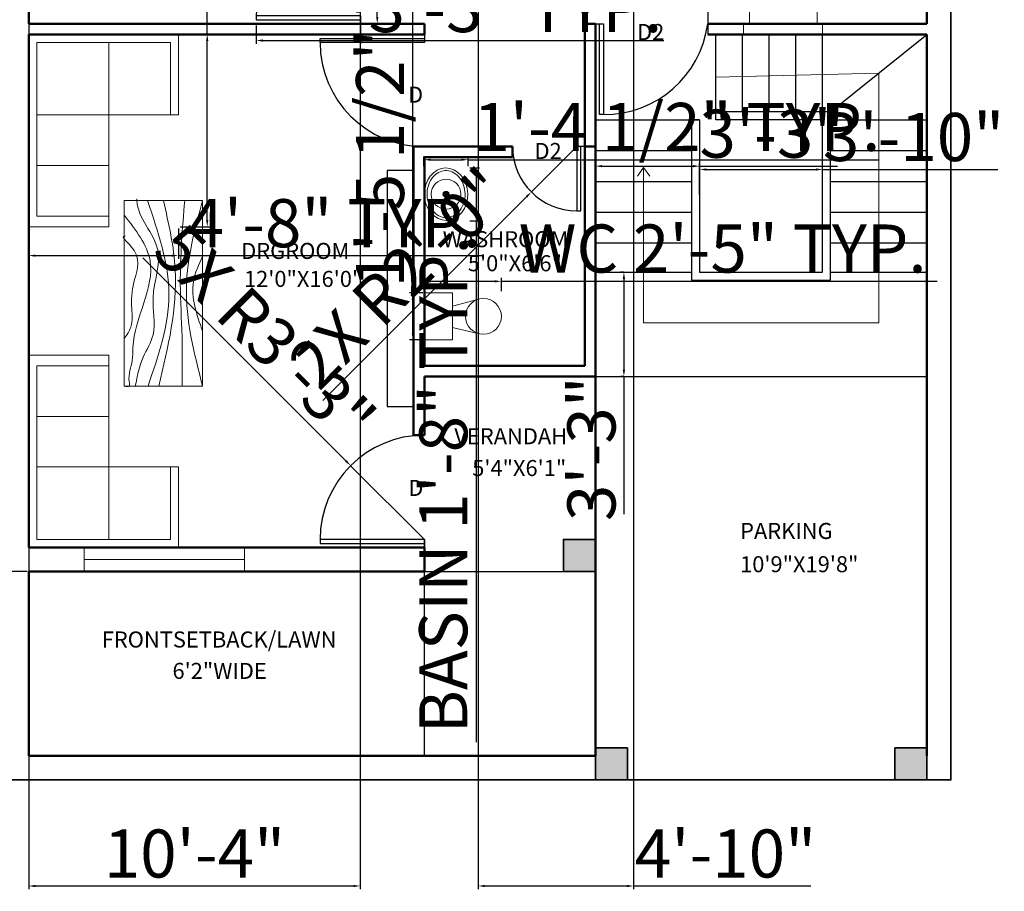
# Model space of a CAD drawing. Units: inches. Extents: x 2040 to 2729, y 1653 to 2621.
# Tile 2 of 4: x 2273 to 2641, y 1653 to 1979. Entities that reach past the tile are written whole.
import ezdxf

# ---------------------------------------------------------------- set-up
doc = ezdxf.new("R2010")
doc.units = ezdxf.units.IN
doc.layers.get('0').update_dxf_attribs({"color": 111})
for name, color, linetype, lineweight in [('A-ANNO-DIMS', 10, 'Continuous', 18), ('A-ANNO-SYMB', 10, 'Continuous', 18), ('A-ANNO-TEXT', 30, 'Continuous', 18), ('A-AREA-IDEN', 6, 'Continuous', 18), ('A-COLS', 7, 'Continuous', 35), ('A-COLS-PATT', 1, 'Continuous', 13), ('A-DOOR', 50, 'Continuous', 25), ('A-EQPM', 8, 'Continuous', 18), ('A-FLOR-CASE', 30, 'Continuous', 25), ('A-FLOR-FIXT', 4, 'Continuous', 18), ('A-FLOR-OTLN', 111, 'Continuous', 25), ('A-FLOR-STRS', 50, 'Continuous', 25), ('A-FURN', 30, 'Continuous', 18), ('A-GLAZ', 31, 'Continuous', 18), ('A-WALL', 7, 'Continuous', 50), ('C-PROP', 111, 'Continuous', 35)]:
    doc.layers.add(name, color=color, linetype=linetype, lineweight=lineweight)
doc.styles.get("Standard").update_dxf_attribs({"font": 'arial.ttf'})
doc.dimstyles.new('ISO-25', dxfattribs={"dimtxt": 18, "dimasz": 2.5, "dimexe": 1.25, "dimexo": 0.625, "dimtad": 1, "dimdec": 0, "dimlunit": 3, "dimtxsty": 'Standard', "dimcen": 2.5, "dimadec": 0, "dimazin": 0, "dimtfac": 1, "dimtdec": 0, "dimtmove": 0, "dimatfit": 3, "dimfxl": 1, "dimarcsym": 0})

# ---------------------------------------------------------------- blocks, each defined once
blk = doc.blocks.new('*D2')
at = {"layer": 'A-ANNO-DIMS', "color": 0, "lineweight": -2, "transparency": 16777216}
for p, q in [((2527.47, 1913.79), (2527.47, 1924.35)), ((2529.97, 1923.1), (2570.97, 1923.1)), ((2573.47, 1913.79), (2573.47, 1924.35)), ((2573.47, 1923.1), (2639.04, 1923.1))]:
    blk.add_line(p, q, dxfattribs=at)
at = {"layer": 'A-ANNO-DIMS', "color": 0, "transparency": 16777216}
for points in [[(2529.97, 1923.51), (2529.97, 1922.68), (2527.47, 1923.1)], [(2570.97, 1923.51), (2570.97, 1922.68), (2573.47, 1923.1)]]:
    blk.add_solid(points, dxfattribs=at)
at = {"layer": 'Defpoints', "color": 0, "transparency": 16777216}
for p in [(2573.47, 1923.1), (2527.47, 1913.16), (2573.47, 1913.16)]:
    blk.add_point(p, dxfattribs=at)
at = {"layer": 'A-ANNO-DIMS', "color": 0, "transparency": 16777216, "insert": (2607.51, 1932.92), "char_height": 18, "attachment_point": 5}
blk.add_mtext('3\'-10"', dxfattribs=at)
blk = doc.blocks.new('*D3')
at = {"layer": 'A-ANNO-DIMS', "color": 0, "lineweight": -2, "transparency": 16777216}
for p, q in [((2488.47, 1923.72), (2488.47, 1925.6)), ((2490.97, 1924.35), (2524.97, 1924.35)), ((2527.47, 1923.72), (2527.47, 1925.6)), ((2527.47, 1924.35), (2579.06, 1924.35))]:
    blk.add_line(p, q, dxfattribs=at)
at = {"layer": 'A-ANNO-DIMS', "color": 0, "transparency": 16777216}
for points in [[(2490.97, 1924.76), (2490.97, 1923.93), (2488.47, 1924.35)], [(2524.97, 1924.76), (2524.97, 1923.93), (2527.47, 1924.35)]]:
    blk.add_solid(points, dxfattribs=at)
at = {"layer": 'Defpoints', "color": 0, "transparency": 16777216}
for p in [(2488.47, 1923.1), (2527.47, 1924.35), (2527.47, 1923.1)]:
    blk.add_point(p, dxfattribs=at)
at = {"layer": 'A-ANNO-DIMS', "color": 0, "transparency": 16777216, "insert": (2554.52, 1934.17), "char_height": 18, "attachment_point": 5}
blk.add_mtext('3\'-3"', dxfattribs=at)
blk = doc.blocks.new('*D4')
at = {"layer": 'A-ANNO-DIMS', "color": 0, "lineweight": -2, "transparency": 16777216}
for p, q in [((2498.94, 1884.66), (2497.88, 1884.66)), ((2499.13, 1882.16), (2499.13, 1848.16)), ((2498.94, 1845.66), (2497.88, 1845.66)), ((2499.13, 1845.66), (2499.13, 1794.07))]:
    blk.add_line(p, q, dxfattribs=at)
at = {"layer": 'A-ANNO-DIMS', "color": 0, "transparency": 16777216}
for points in [[(2498.72, 1882.16), (2499.55, 1882.16), (2499.13, 1884.66)], [(2498.72, 1848.16), (2499.55, 1848.16), (2499.13, 1845.66)]]:
    blk.add_solid(points, dxfattribs=at)
at = {"layer": 'Defpoints', "color": 0, "transparency": 16777216}
for p in [(2499.56, 1884.66), (2499.13, 1845.66), (2499.56, 1845.66)]:
    blk.add_point(p, dxfattribs=at)
at = {"layer": 'A-ANNO-DIMS', "color": 0, "transparency": 16777216, "insert": (2489.31, 1818.62), "char_height": 18, "attachment_point": 5, "rotation": 90}
blk.add_mtext('3\'-3"', dxfattribs=at)
blk = doc.blocks.new('WC-FLOOR-MOUNT')
for p, q in [((0, 0), (10.48, 0)), ((0, -17.59), (0, 0)), ((10.48, 0), (10.48, -17.59)), ((10.48, -5), (20.35, -2.32)), ((10.48, -12.9), (20.54, -15.32)), ((10.48, -17.59), (0, -17.59))]:
    blk.add_line(p, q)
blk.add_circle((22.11, -8.8), 6.71)
blk = doc.blocks.new('BASIN-OVAL')
h = blk.add_hatch(color=256)
h.dxf.hatch_style = 1
h.paths.add_polyline_path([(1.14, 0, 1), (-1.14, 0, 1)])
for radius in [5.58, 1.14]:
    blk.add_circle((0, 0), radius)
blk.add_ellipse((0, 0), major_axis=(9.81, 0.23), ratio=0.826688)
blk.add_open_spline([(8.81, 0.21), (8.8, 0.81), (8.69, 1.4), (8.2, 2.81), (7.72, 3.6), (6.41, 5.01), (5.59, 5.62), (3.7, 6.55), (2.64, 6.87), (0.44, 7.17), (-0.7, 7.15), (-2.89, 6.76), (-3.94, 6.39), (-5.79, 5.39), (-6.59, 4.75), (-7.85, 3.29), (-8.3, 2.48), (-8.82, 0.79), (-8.88, -0.08), (-8.62, -1.78), (-8.3, -2.62), (-7.28, -4.16), (-6.59, -4.86), (-4.92, -6.01), (-3.94, -6.46), (-1.83, -7.03), (-0.7, -7.16), (1.53, -7.05), (2.64, -6.83), (4.67, -6.06), (5.59, -5.52), (7.11, -4.23), (7.72, -3.47), (8.55, -1.86), (8.78, -1), (8.82, -0.02), (8.82, 0.09), (8.81, 0.21)], degree=3, knots=[0, 0, 0, 0, 0.259704, 0.259704, 0.633026, 0.633026, 1.006347, 1.006347, 1.379668, 1.379668, 1.752989, 1.752989, 2.12631, 2.12631, 2.499631, 2.499631, 2.872952, 2.872952, 3.246274, 3.246274, 3.619595, 3.619595, 3.992916, 3.992916, 4.366237, 4.366237, 4.739558, 4.739558, 5.112879, 5.112879, 5.486201, 5.486201, 5.859522, 5.859522, 6.232843, 6.232843, 6.283185, 6.283185, 6.283185, 6.283185])
blk = doc.blocks.new('SOFA-CORNER')
for p, q in [((0, 30.1), (-55.97, 30.1)), ((-55.97, 30.1), (-55.97, -41.9)), ((0, 0), (0, 30.1)), ((-52.97, -37.9), (-52.97, 27.1)), ((-52.97, 27.1), (-2.97, 27.1)), ((-25.97, 0), (-25.97, 27.1)), ((-2.97, 27.1), (-2.97, 0)), ((-2.97, 0), (-52.97, 0)), ((-25.97, -37.9), (-25.97, 0)), ((-2.97, 0), (0, 0)), ((-25.97, -18.95), (-52.97, -18.95)), ((-25.97, -37.9), (-52.97, -37.9)), ((-25.97, -41.9), (-25.97, -37.9)), ((-55.97, -41.9), (-25.97, -41.9))]:
    blk.add_line(p, q)
blk = doc.blocks.new('DOOR-39IN')
for p, q in [((0, 0), (0, 39)), ((0, 39), (1.5, 39)), ((1.5, 39), (1.5, 0)), ((3, 0), (0, 0))]:
    blk.add_line(p, q)
blk.add_arc((0, 0), 39, 90, 180)
blk = doc.blocks.new('DOOR-39IN-ALT')
for p, q in [((0, 0), (-39, 0)), ((-39, 0), (-39, -1.5)), ((0, 0), (0, -3)), ((0, -3), (0, 0)), ((-39, -1.5), (0, -1.5)), ((-39, -1.5), (0, -1.5))]:
    blk.add_line(p, q)
blk.add_arc((0, 0), 39, 90, 180)
blk = doc.blocks.new('*D19')
at = {"layer": 'A-ANNO-DIMS', "color": 0, "lineweight": -2, "transparency": 16777216}
for p, q in [((2441.45, 1923.78), (2445.06, 1923.78)), ((2443.81, 1921.28), (2443.81, 1906.43)), ((2441.45, 1903.93), (2445.06, 1903.93)), ((2443.81, 1903.93), (2443.81, 1708.82))]:
    blk.add_line(p, q, dxfattribs=at)
at = {"layer": 'A-ANNO-DIMS', "color": 0, "transparency": 16777216}
for points in [[(2443.39, 1921.28), (2444.22, 1921.28), (2443.81, 1923.78)], [(2443.39, 1906.43), (2444.22, 1906.43), (2443.81, 1903.93)]]:
    blk.add_solid(points, dxfattribs=at)
at = {"layer": 'Defpoints', "color": 0, "transparency": 16777216}
for p in [(2440.83, 1923.78), (2440.83, 1903.93), (2443.81, 1903.93)]:
    blk.add_point(p, dxfattribs=at)
at = {"layer": 'A-ANNO-DIMS', "color": 0, "transparency": 16777216, "insert": (2433.87, 1805.12), "char_height": 18, "attachment_point": 5, "rotation": 90}
blk.add_mtext('BASIN 1\'-8" TYP.', dxfattribs=at)
blk = doc.blocks.new('*D20')
at = {"layer": 'A-ANNO-DIMS', "color": 0, "lineweight": -2, "transparency": 16777216}
for p, q in [((2424.34, 1924.4), (2424.34, 1928)), ((2426.84, 1926.75), (2438.33, 1926.75)), ((2440.83, 1924.4), (2440.83, 1928)), ((2440.83, 1926.75), (2594.55, 1926.75))]:
    blk.add_line(p, q, dxfattribs=at)
at = {"layer": 'A-ANNO-DIMS', "color": 0, "transparency": 16777216}
for points in [[(2426.84, 1927.17), (2426.84, 1926.34), (2424.34, 1926.75)], [(2438.33, 1927.17), (2438.33, 1926.34), (2440.83, 1926.75)]]:
    blk.add_solid(points, dxfattribs=at)
at = {"layer": 'Defpoints', "color": 0, "transparency": 16777216}
for p in [(2440.83, 1926.75), (2424.34, 1923.78), (2440.83, 1923.78)]:
    blk.add_point(p, dxfattribs=at)
at = {"layer": 'A-ANNO-DIMS', "color": 0, "transparency": 16777216, "insert": (2518.94, 1936.69), "char_height": 18, "attachment_point": 5}
blk.add_mtext('1\'-4 1/2" TYP.', dxfattribs=at)
blk = doc.blocks.new('*D23')
at = {"layer": 'A-ANNO-DIMS', "color": 0, "lineweight": -2, "transparency": 16777216}
for p, q in [((2424.47, 1877.55), (2424.47, 1882.49)), ((2453.3, 1877.55), (2453.3, 1882.49)), ((2426.97, 1881.24), (2450.8, 1881.24)), ((2453.3, 1881.24), (2616.39, 1881.24))]:
    blk.add_line(p, q, dxfattribs=at)
at = {"layer": 'A-ANNO-DIMS', "color": 0, "transparency": 16777216}
for points in [[(2426.97, 1881.66), (2426.97, 1880.83), (2424.47, 1881.24)], [(2450.8, 1881.66), (2450.8, 1880.83), (2453.3, 1881.24)]]:
    blk.add_solid(points, dxfattribs=at)
at = {"layer": 'Defpoints', "color": 0, "transparency": 16777216}
for p in [(2453.3, 1881.24), (2424.47, 1876.92), (2453.3, 1876.92)]:
    blk.add_point(p, dxfattribs=at)
at = {"layer": 'A-ANNO-DIMS', "color": 0, "transparency": 16777216, "insert": (2536.09, 1891.18), "char_height": 18, "attachment_point": 5}
blk.add_mtext('WC 2\'-5" TYP.', dxfattribs=at)
blk = doc.blocks.new('*D24')
at = {"layer": 'A-ANNO-DIMS', "color": 0, "lineweight": -2, "transparency": 16777216}
for p, q in [((2420.15, 1876.92), (2420.15, 2030.64)), ((2423.85, 1876.92), (2418.9, 1876.92)), ((2420.15, 1861.83), (2420.15, 1874.42)), ((2423.85, 1859.33), (2418.9, 1859.33))]:
    blk.add_line(p, q, dxfattribs=at)
at = {"layer": 'A-ANNO-DIMS', "color": 0, "transparency": 16777216}
for points in [[(2419.73, 1874.42), (2420.57, 1874.42), (2420.15, 1876.92)], [(2419.73, 1861.83), (2420.57, 1861.83), (2420.15, 1859.33)]]:
    blk.add_solid(points, dxfattribs=at)
at = {"layer": 'Defpoints', "color": 0, "transparency": 16777216}
for p in [(2420.15, 1876.92), (2424.47, 1876.92), (2424.47, 1859.33)]:
    blk.add_point(p, dxfattribs=at)
at = {"layer": 'A-ANNO-DIMS', "color": 0, "transparency": 16777216, "insert": (2410.22, 1955.03), "char_height": 18, "attachment_point": 5, "rotation": 90}
blk.add_mtext('1\'-5 1/2" TYP.', dxfattribs=at)
blk = doc.blocks.new('*D29')
at = {"layer": 'A-ANNO-DIMS', "color": 0, "lineweight": -2, "transparency": 16777216}
for p, q in [((2343.24, 1973.66), (2343.24, 2162.49)), ((2333.07, 1973.66), (2344.49, 1973.66)), ((2343.24, 1904.16), (2343.24, 1971.16)), ((2333.07, 1901.66), (2344.49, 1901.66))]:
    blk.add_line(p, q, dxfattribs=at)
at = {"layer": 'A-ANNO-DIMS', "color": 0, "transparency": 16777216}
for points in [[(2342.83, 1971.16), (2343.66, 1971.16), (2343.24, 1973.66)], [(2342.83, 1904.16), (2343.66, 1904.16), (2343.24, 1901.66)]]:
    blk.add_solid(points, dxfattribs=at)
at = {"layer": 'Defpoints', "color": 0, "transparency": 16777216}
for p in [(2332.44, 1973.66), (2343.24, 1973.66), (2332.44, 1901.66)]:
    blk.add_point(p, dxfattribs=at)
at = {"layer": 'A-ANNO-DIMS', "color": 0, "transparency": 16777216, "insert": (2333.3, 2069.33), "char_height": 18, "attachment_point": 5, "rotation": 90}
blk.add_mtext('SOFA 6\'-0" TYP.', dxfattribs=at)
blk = doc.blocks.new('*D30')
at = {"layer": 'A-ANNO-DIMS', "color": 0, "lineweight": -2, "transparency": 16777216}
for p, q in [((2276.47, 1901.04), (2276.47, 1889.61)), ((2332.44, 1901.04), (2332.44, 1889.61)), ((2278.97, 1890.86), (2329.94, 1890.86)), ((2332.44, 1890.86), (2446.64, 1890.86))]:
    blk.add_line(p, q, dxfattribs=at)
at = {"layer": 'A-ANNO-DIMS', "color": 0, "transparency": 16777216}
for points in [[(2278.97, 1891.28), (2278.97, 1890.44), (2276.47, 1890.86)], [(2329.94, 1891.28), (2329.94, 1890.44), (2332.44, 1890.86)]]:
    blk.add_solid(points, dxfattribs=at)
at = {"layer": 'Defpoints', "color": 0, "transparency": 16777216}
for p in [(2276.47, 1901.66), (2332.44, 1901.66), (2332.44, 1890.86)]:
    blk.add_point(p, dxfattribs=at)
at = {"layer": 'A-ANNO-DIMS', "color": 0, "transparency": 16777216, "insert": (2390.79, 1900.68), "char_height": 18, "attachment_point": 5}
blk.add_mtext('4\'-8" TYP.', dxfattribs=at)
blk = doc.blocks.new('*D33')
at = {"layer": 'A-ANNO-DIMS', "color": 0, "lineweight": -2, "transparency": 16777216}
for p, q in [((2406.86, 2019.66), (2406.86, 2351.67)), ((2401.19, 2019.66), (2408.11, 2019.66)), ((2406.86, 1980.16), (2406.86, 2017.16)), ((2401.19, 1977.66), (2408.11, 1977.66))]:
    blk.add_line(p, q, dxfattribs=at)
at = {"layer": 'A-ANNO-DIMS', "color": 0, "transparency": 16777216}
for points in [[(2406.45, 2017.16), (2407.28, 2017.16), (2406.86, 2019.66)], [(2406.45, 1980.16), (2407.28, 1980.16), (2406.86, 1977.66)]]:
    blk.add_solid(points, dxfattribs=at)
at = {"layer": 'Defpoints', "color": 0, "transparency": 16777216}
for p in [(2400.56, 2019.66), (2406.86, 2019.66), (2400.56, 1977.66)]:
    blk.add_point(p, dxfattribs=at)
at = {"layer": 'A-ANNO-DIMS', "color": 0, "transparency": 16777216, "insert": (2396.92, 2186.92), "char_height": 18, "attachment_point": 5, "rotation": 90}
blk.add_mtext('BEDROOM DOOR 3\'-6" TYP.', dxfattribs=at)
blk = doc.blocks.new('*D34')
at = {"layer": 'A-ANNO-DIMS', "color": 0, "lineweight": -2, "transparency": 16777216}
for p, q in [((2361.56, 1977.04), (2361.56, 1970.11)), ((2400.56, 1977.04), (2400.56, 1970.11)), ((2364.06, 1971.36), (2398.06, 1971.36)), ((2400.56, 1971.36), (2514.02, 1971.36))]:
    blk.add_line(p, q, dxfattribs=at)
at = {"layer": 'A-ANNO-DIMS', "color": 0, "transparency": 16777216}
for points in [[(2364.06, 1971.78), (2364.06, 1970.94), (2361.56, 1971.36)], [(2398.06, 1971.78), (2398.06, 1970.94), (2400.56, 1971.36)]]:
    blk.add_solid(points, dxfattribs=at)
at = {"layer": 'Defpoints', "color": 0, "transparency": 16777216}
for p in [(2361.56, 1977.66), (2400.56, 1977.66), (2400.56, 1971.36)]:
    blk.add_point(p, dxfattribs=at)
at = {"layer": 'A-ANNO-DIMS', "color": 0, "transparency": 16777216, "insert": (2458.54, 1981.18), "char_height": 18, "attachment_point": 5}
blk.add_mtext('3\'-3" TYP.', dxfattribs=at)
blk = doc.blocks.new('*D41')
at = {"layer": 'A-ANNO-DIMS', "color": 0, "lineweight": -2, "transparency": 16777216}
for p, q in [((2266.85, 2402.66), (2226.49, 2402.66)), ((2227.74, 1775.16), (2227.74, 2400.16)), ((2275.85, 1772.66), (2226.49, 1772.66))]:
    blk.add_line(p, q, dxfattribs=at)
at = {"layer": 'A-ANNO-DIMS', "color": 0, "transparency": 16777216}
for points in [[(2227.33, 2400.16), (2228.16, 2400.16), (2227.74, 2402.66)], [(2227.33, 1775.16), (2228.16, 1775.16), (2227.74, 1772.66)]]:
    blk.add_solid(points, dxfattribs=at)
at = {"layer": 'Defpoints', "color": 0, "transparency": 16777216}
for p in [(2227.74, 2402.66), (2267.47, 2402.66), (2276.47, 1772.66)]:
    blk.add_point(p, dxfattribs=at)
at = {"layer": 'A-ANNO-DIMS', "color": 0, "transparency": 16777216, "insert": (2217.93, 2087.66), "char_height": 18, "attachment_point": 5, "rotation": 90}
blk.add_mtext('52\'-6"', dxfattribs=at)
blk = doc.blocks.new('*D44')
at = {"layer": 'A-ANNO-DIMS', "color": 0, "lineweight": -2, "transparency": 16777216}
for p, q in [((2276.47, 2169.04), (2276.47, 1653.68)), ((2400.47, 2169.04), (2400.47, 1653.68)), ((2278.97, 1654.93), (2397.97, 1654.93))]:
    blk.add_line(p, q, dxfattribs=at)
at = {"layer": 'A-ANNO-DIMS', "color": 0, "transparency": 16777216}
for points in [[(2278.97, 1655.35), (2278.97, 1654.51), (2276.47, 1654.93)], [(2397.97, 1655.35), (2397.97, 1654.51), (2400.47, 1654.93)]]:
    blk.add_solid(points, dxfattribs=at)
at = {"layer": 'Defpoints', "color": 0, "transparency": 16777216}
for p in [(2276.47, 2169.66), (2400.47, 2169.66), (2400.47, 1654.93)]:
    blk.add_point(p, dxfattribs=at)
at = {"layer": 'A-ANNO-DIMS', "color": 0, "transparency": 16777216, "insert": (2338.47, 1664.75), "char_height": 18, "attachment_point": 5}
blk.add_mtext('10\'-4"', dxfattribs=at)
blk = doc.blocks.new('*D45')
at = {"layer": 'A-ANNO-DIMS', "color": 0, "lineweight": -2, "transparency": 16777216}
for p, q in [((2444.6, 2057.89), (2444.6, 1653.68)), ((2502.75, 2057.89), (2502.75, 1653.68)), ((2447.1, 1654.93), (2500.25, 1654.93)), ((2502.75, 1654.93), (2569.05, 1654.93))]:
    blk.add_line(p, q, dxfattribs=at)
at = {"layer": 'A-ANNO-DIMS', "color": 0, "transparency": 16777216}
for points in [[(2447.1, 1655.35), (2447.1, 1654.51), (2444.6, 1654.93)], [(2500.25, 1655.35), (2500.25, 1654.51), (2502.75, 1654.93)]]:
    blk.add_solid(points, dxfattribs=at)
at = {"layer": 'Defpoints', "color": 0, "transparency": 16777216}
for p in [(2444.6, 2058.52), (2502.75, 2058.52), (2502.75, 1654.93)]:
    blk.add_point(p, dxfattribs=at)
at = {"layer": 'A-ANNO-DIMS', "color": 0, "transparency": 16777216, "insert": (2537.15, 1664.75), "char_height": 18, "attachment_point": 5}
blk.add_mtext('4\'-10"', dxfattribs=at)
blk = doc.blocks.new('*D48')
at = {"layer": 'A-ANNO-DIMS', "color": 0, "lineweight": -2, "transparency": 16777216}
for p, q in [((2481.47, 1931.66), (2464.5, 1914.69)), ((2386.5, 1836.69), (2462.74, 1912.92))]:
    blk.add_line(p, q, dxfattribs=at)
at = {"layer": 'A-ANNO-DIMS', "color": 0, "transparency": 16777216}
blk.add_solid([(2462.44, 1913.22), (2463.03, 1912.63), (2464.5, 1914.69)], dxfattribs=at)
at = {"layer": 'Defpoints', "color": 0, "transparency": 16777216}
for p in [(2481.47, 1931.66), (2464.5, 1914.69)]:
    blk.add_point(p, dxfattribs=at)
at = {"layer": 'A-ANNO-DIMS', "color": 0, "transparency": 16777216, "insert": (2416.79, 1880.86), "char_height": 18, "attachment_point": 5, "rotation": 44.9992}
blk.add_mtext('2X R2\'-0"', dxfattribs=at)
blk = doc.blocks.new('*D52')
at = {"layer": 'A-ANNO-DIMS', "color": 0, "lineweight": -2, "transparency": 16777216}
for p, q in [((2319.12, 1890.03), (2395.13, 1814.01)), ((2424.47, 1784.66), (2396.9, 1812.24))]:
    blk.add_line(p, q, dxfattribs=at)
at = {"layer": 'A-ANNO-DIMS', "color": 0, "transparency": 16777216}
blk.add_solid([(2395.43, 1814.3), (2394.84, 1813.71), (2396.9, 1812.24)], dxfattribs=at)
at = {"layer": 'Defpoints', "color": 0, "transparency": 16777216}
for p in [(2396.9, 1812.24), (2424.47, 1784.66)]:
    blk.add_point(p, dxfattribs=at)
at = {"layer": 'A-ANNO-DIMS', "color": 0, "transparency": 16777216, "insert": (2363.19, 1859.85), "char_height": 18, "attachment_point": 5, "rotation": 314.9947}
blk.add_mtext('5X R3\'-3"', dxfattribs=at)

msp = doc.modelspace()

# ---------------------------------------------------------------- hatches: boundary and pattern name
at = {"layer": 'A-COLS-PATT'}
h = msp.add_hatch(color=256, dxfattribs=at)
h.dxf.hatch_style = 1
h.paths.add_polyline_path([(2488.47, 1784.66), (2476.47, 1784.66), (2476.47, 1772.66), (2488.47, 1772.66)])
h = msp.add_hatch(color=256, dxfattribs=at)
h.dxf.hatch_style = 1
h.paths.add_polyline_path([(2500.47, 1706.66), (2488.47, 1706.66), (2488.47, 1703.66), (2488.47, 1694.66), (2500.47, 1694.66)])
h = msp.add_hatch(color=256, dxfattribs=at)
h.dxf.hatch_style = 1
h.paths.add_polyline_path([(2612.47, 1703.66), (2612.47, 1706.66), (2600.47, 1706.66), (2600.47, 1694.66), (2612.47, 1694.66)])

# ---------------------------------------------------------------- linework, layer by layer
at = {"layer": 'A-ANNO-SYMB'}
for p, q in [((2533.47, 1957.66), (2594.47, 1959.16)), ((2594.47, 1959.16), (2594.47, 1865.68)), ((2506.47, 1923.9), (2504.18, 1920.62)), ((2506.47, 1865.68), (2506.47, 1923.9)), ((2506.47, 1923.9), (2508.77, 1920.62)), ((2594.47, 1865.68), (2506.47, 1865.68))]:
    msp.add_line(p, q, dxfattribs=at)
at = {"layer": 'A-COLS'}
for p, q in [((2500.47, 1706.66), (2488.47, 1706.66)), ((2500.47, 1694.66), (2500.47, 1706.66)), ((2600.47, 1694.66), (2600.47, 1706.66)), ((2600.47, 1706.66), (2612.47, 1706.66)), ((2488.47, 1703.66), (2488.47, 1694.66)), ((2612.47, 1703.66), (2612.47, 1694.66)), ((2488.47, 1694.66), (2500.47, 1694.66)), ((2612.47, 1694.66), (2600.47, 1694.66))]:
    msp.add_line(p, q, dxfattribs=at)
msp.add_lwpolyline([(2488.47, 1772.66), (2476.47, 1772.66), (2476.47, 1784.66), (2488.47, 1784.66)], close=True, dxfattribs=at)
at = {"layer": 'A-DOOR'}
for p, q in [((2488.47, 1977.66), (2491.47, 1977.66)), ((2489.97, 1943.66), (2489.97, 1977.66)), ((2491.47, 1977.66), (2491.47, 1943.66)), ((2491.47, 1943.66), (2489.97, 1943.66)), ((2484.47, 1931.66), (2481.47, 1931.66)), ((2481.47, 1931.66), (2481.47, 1907.66)), ((2482.97, 1907.66), (2482.97, 1931.66)), ((2481.47, 1907.66), (2482.97, 1907.66))]:
    msp.add_line(p, q, dxfattribs=at)
for centre, radius, start, end in [((2491.8, 1982.66), 39, 269.5274, 352.6361), ((2481.47, 1931.66), 24, 180, 270)]:
    msp.add_arc(centre, radius, start, end, dxfattribs=at)
at = {"layer": 'A-EQPM'}
msp.add_lwpolyline([(2571.47, 1977.66), (2546.15, 1977.66), (2546.15, 2001.66), (2571.47, 2001.66)], close=True, dxfattribs=at)
at = {"layer": 'A-FLOR-CASE'}
msp.add_line((2530.47, 2001.66), (2530.47, 1973.66), dxfattribs=at)
msp.add_lwpolyline([(2420.47, 1922.66), (2410.6, 1922.66), (2410.6, 1834.33), (2420.47, 1834.33)], close=True, dxfattribs=at)
at = {"layer": 'A-FLOR-OTLN'}
for p, q in [((2424.47, 1703.66), (2424.47, 1772.66)), ((2424.47, 1772.66), (2488.47, 1772.66))]:
    msp.add_line(p, q, dxfattribs=at)
at = {"layer": 'A-FLOR-STRS'}
for p, q in [((2533.47, 1941.66), (2533.47, 1973.66)), ((2543.47, 1944.66), (2543.47, 1973.66)), ((2553.47, 1944.66), (2553.47, 1973.66)), ((2563.47, 1944.66), (2563.47, 1973.66)), ((2573.47, 1944.66), (2573.47, 1973.66)), ((2576.47, 1944.66), (2612.47, 1973.66)), ((2488.47, 1941.66), (2527.47, 1941.66)), ((2527.47, 1941.66), (2524.47, 1941.66)), ((2524.47, 1941.66), (2524.47, 1881.66)), ((2527.47, 1941.66), (2527.47, 1884.66)), ((2576.47, 1944.66), (2533.47, 1944.66)), ((2573.47, 1941.66), (2533.47, 1941.66)), ((2573.47, 1884.66), (2573.47, 1941.66)), ((2576.47, 1881.66), (2576.47, 1944.66)), ((2576.47, 1941.66), (2612.47, 1941.66)), ((2488.47, 1930.16), (2524.47, 1930.16)), ((2576.47, 1930.16), (2612.47, 1930.16)), ((2488.47, 1918.66), (2524.47, 1918.66)), ((2576.47, 1918.66), (2612.47, 1918.66)), ((2488.47, 1907.16), (2524.47, 1907.16)), ((2576.47, 1907.16), (2612.47, 1907.16)), ((2488.47, 1895.66), (2524.47, 1895.66)), ((2576.47, 1895.66), (2612.47, 1895.66)), ((2488.47, 1884.66), (2524.47, 1884.66)), ((2527.47, 1884.66), (2573.47, 1884.66)), ((2576.47, 1884.66), (2612.47, 1884.66)), ((2524.47, 1881.66), (2576.47, 1881.66)), ((2488.47, 1845.66), (2612.47, 1845.66))]:
    msp.add_line(p, q, dxfattribs=at)
at = {"layer": 'A-FURN'}
msp.add_line((2332.44, 1781.66), (2276.47, 1781.66), dxfattribs=at)
msp.add_lwpolyline([(2312.21, 1911.49), (2341.5, 1911.49), (2341.5, 1842.04), (2312.21, 1842.04)], close=True, dxfattribs=at)
for points, knots in [([(2316.32, 1842.04), (2317.07, 1845.73), (2318.42, 1852.4), (2324.92, 1862.47), (2321.12, 1876.55), (2329.02, 1894.28), (2316.88, 1905.01), (2316.95, 1911.91), (2316.95, 1912.13)], [0, 0, 0, 0, 11.286534, 20.351276, 34.306788, 52.246482, 72.293035, 72.936945, 72.936945, 72.936945, 72.936945]), ([(2320.85, 1911.49), (2324.89, 1899.76), (2332.87, 1876.61), (2324.99, 1853.46), (2321.1, 1842.04)], [0, 0, 0, 0, 36.097508, 71.234431, 71.234431, 71.234431, 71.234431]), ([(2326.85, 1911.49), (2328.84, 1902.86), (2334.15, 1879.8), (2328.6, 1856.58), (2325.13, 1842.04)], [0, 0, 0, 0, 26.261914, 70.259672, 70.259672, 70.259672, 70.259672]), ([(2334.82, 1911.49), (2333.96, 1901.1), (2332.56, 1884.14), (2334.04, 1860.98), (2333.89, 1848.22), (2333.81, 1842.04)], [0, 0, 0, 0, 31.207497, 50.956396, 69.500686, 69.500686, 69.500686, 69.500686]), ([(2341.5, 1911.49), (2338.6, 1900.73), (2332.38, 1877.65), (2338.32, 1854.43), (2341.5, 1842.04)], [0, 0, 0, 0, 32.857913, 70.498944, 70.498944, 70.498944, 70.498944]), ([(2312.21, 1905.97), (2316.51, 1900.44), (2328.12, 1885.51), (2314.88, 1866.09), (2315.54, 1850.39), (2313.37, 1846.4), (2314.49, 1841.56), (2312.99, 1841.87), (2312.21, 1842.04)], [0, 0, 0, 0, 19.52057, 52.709722, 57.61946, 65.496264, 67.193354, 69.034395, 69.034395, 69.034395, 69.034395]), ([(2312.21, 1859.83), (2313.2, 1861.21), (2315.79, 1864.84), (2314.46, 1872.84), (2315.8, 1883.1), (2319.4, 1890.8), (2310.78, 1898.23), (2312.43, 1898.18), (2312.54, 1898.17)], [0, 0, 0, 0, 4.937051, 12.987406, 22.85915, 35.522025, 39.856714, 40.187852, 40.187852, 40.187852, 40.187852]), ([(2341.5, 1890.63), (2340.06, 1887.51), (2335.91, 1878.51), (2339.29, 1868.88), (2341.5, 1862.59)], [0, 0, 0, 0, 10.026259, 28.943072, 28.943072, 28.943072, 28.943072])]:
    msp.add_open_spline(points, degree=3, knots=knots, dxfattribs=at)
at = {"layer": 'A-GLAZ'}
msp.add_line((2297.24, 1777.16), (2357.24, 1777.16), dxfattribs=at)
for points in [[(2543.91, 1977.66), (2573.47, 1977.66), (2573.47, 1973.66), (2543.91, 1973.66)], [(2297.24, 1781.66), (2357.24, 1781.66), (2357.24, 1772.66), (2297.24, 1772.66)]]:
    msp.add_lwpolyline(points, close=True, dxfattribs=at)
at = {"layer": 'A-WALL'}
for p, q in [((2276.47, 1977.66), (2276.47, 2393.66)), ((2612.47, 2121.66), (2612.47, 1977.66)), ((2276.47, 1977.66), (2424.47, 1977.66)), ((2424.47, 1973.66), (2424.47, 1977.66)), ((2484.47, 1849.66), (2484.47, 1977.66)), ((2484.47, 1977.66), (2488.47, 1977.66)), ((2488.47, 1703.66), (2488.47, 1977.66)), ((2530.47, 1977.66), (2612.47, 1977.66)), ((2276.47, 1973.66), (2424.47, 1973.66)), ((2276.47, 1781.66), (2276.47, 1973.66)), ((2530.47, 1973.66), (2612.47, 1973.66)), ((2612.47, 1973.66), (2612.47, 1703.66)), ((2420.47, 1931.66), (2457.47, 1931.66)), ((2420.47, 1922.66), (2420.47, 1931.66)), ((2457.47, 1931.66), (2457.47, 1927.66)), ((2484.47, 1931.66), (2488.47, 1931.66)), ((2424.47, 1927.66), (2457.47, 1927.66)), ((2424.47, 1918.66), (2424.47, 1927.66)), ((2420.47, 1823.66), (2420.47, 1922.66)), ((2424.47, 1849.66), (2424.47, 1918.66)), ((2424.47, 1849.66), (2484.47, 1849.66)), ((2424.47, 1823.66), (2424.47, 1845.66)), ((2424.47, 1845.66), (2488.47, 1845.66)), ((2424.47, 1823.66), (2420.47, 1823.66)), ((2276.47, 1781.66), (2424.47, 1781.66)), ((2424.47, 1781.66), (2424.47, 1772.66)), ((2276.47, 1703.66), (2276.47, 1772.66)), ((2424.47, 1772.66), (2276.47, 1772.66)), ((2488.47, 1703.66), (2276.47, 1703.66))]:
    msp.add_line(p, q, dxfattribs=at)
at = {"layer": 'C-PROP'}
msp.add_lwpolyline([(2267.47, 2402.66), (2621.47, 2402.66), (2621.47, 1694.66), (2267.47, 1694.66)], close=True, dxfattribs=at)

# ---------------------------------------------------------------- block references
at = {"layer": 'A-DOOR'}
for p in [(2400.56, 1980.66), (2424.47, 1784.66)]:
    msp.add_blockref('DOOR-39IN-ALT', p, dxfattribs=at)
at = {"layer": 'A-DOOR', "rotation": 89.99999999999785}
msp.add_blockref('DOOR-39IN', (2424.47, 1970.66), dxfattribs=at)
at = {"layer": 'A-FLOR-FIXT', "rotation": 269.9999999999998}
msp.add_blockref('BASIN-OVAL', (2432.59, 1913.86), dxfattribs=at)
at = {"layer": 'A-FLOR-FIXT'}
msp.add_blockref('WC-FLOOR-MOUNT', (2424.47, 1876.92), dxfattribs=at)
at = {"layer": 'A-FURN'}
msp.add_blockref('SOFA-CORNER', (2332.44, 1943.56), dxfattribs=at)
at = {"layer": 'A-FURN', "extrusion": (0, 0, -1), "zscale": -1, "rotation": 180}
msp.add_blockref('SOFA-CORNER', (-2332.44, 1811.76), dxfattribs=at)

# ---------------------------------------------------------------- texts
at = {"layer": 'A-ANNO-TEXT'}
for tag, p in [('D2', (2504.06, 1971.54)), ('D', (2418.38, 1948.11)), ('D2', (2465.69, 1927.03)), ('D', (2418.5, 1800.92))]:
    msp.add_attdef(tag, p, '', height=6, dxfattribs=at)
at = {"layer": 'A-AREA-IDEN'}
for tag, p in [('WASHROOM', (2431.34, 1894.01)), ('DRGROOM', (2355.96, 1889.62)), ('5\'0"X6\'6"', (2440.76, 1885.01)), ('12\'0"X16\'0"', (2357, 1879.15)), ('VERANDAH', (2435.7, 1820.27)), ('5\'4"X6\'1"', (2442.38, 1808.36)), ('PARKING', (2542.61, 1784.81)), ('10\'9"X19\'8"', (2542.61, 1772.37)), ('FRONTSETBACK/LAWN', (2303.78, 1744.19)), ('6\'2"WIDE', (2330.24, 1732.44))]:
    msp.add_attdef(tag, p, '', height=6, dxfattribs=at)

# ---------------------------------------------------------------- dimensions: what is measured, and where the dimension line sits
at = {"layer": 'A-ANNO-DIMS'}
for base, p1, p2, override, picture, middle in [((2227.74, 2402.66), (2276.47, 1772.66), (2267.47, 2402.66), {"dimdec": 1, "dimlfac": 1, "dimrnd": 0, "dimzin": 1, "dimdsep": 46, "dimlunit": 4, "dimfrac": 2}, '*D41', (2217.93, 2087.66)), ((2499.13, 1845.66), (2499.56, 1884.66), (2499.56, 1845.66), {"dimclrd": 0, "dimclre": 0, "dimclrt": 0}, '*D4', (2489.31, 1818.62))]:
    dim = msp.add_linear_dim(base=base, p1=p1, p2=p2, angle=90, dimstyle='ISO-25', override=override, dxfattribs=at)
    dim.commit()
    dim.dimension.update_dxf_attribs({"geometry": picture, "text_midpoint": middle})
for base, p1, p2, angle, text, picture, middle in [((2406.86, 2019.66), (2400.56, 1977.66), (2400.56, 2019.66), 90, 'BEDROOM DOOR <> TYP.', '*D33', (2396.92, 2186.92)), ((2343.24, 1973.66), (2332.44, 1901.66), (2332.44, 1973.66), 90, 'SOFA <> TYP.', '*D29', (2333.3, 2069.33)), ((2420.15, 1876.92), (2424.47, 1859.33), (2424.47, 1876.92), 90, '<> TYP.', '*D24', (2410.22, 1955.03)), ((2443.8059, 1903.9348), (2440.8296, 1923.7768), (2440.8296, 1903.9348), 270, 'BASIN <> TYP.', '*D19', (2433.8739, 1805.1249))]:
    dim = msp.add_linear_dim(base=base, p1=p1, p2=p2, angle=angle, text=text, dimstyle='ISO-25', override={"dimdec": 1, "dimlfac": 1, "dimrnd": 0, "dimzin": 1, "dimdsep": 46, "dimlunit": 4, "dimfrac": 2}, dxfattribs=at)
    dim.commit()
    dim.dimension.update_dxf_attribs({"geometry": picture, "text_midpoint": middle})
for base, p1, p2, override, picture, middle in [((2400.47, 1654.93), (2276.47, 2169.66), (2400.47, 2169.66), {"dimdec": 1, "dimlfac": 1, "dimrnd": 0, "dimzin": 1, "dimdsep": 46, "dimlunit": 4, "dimfrac": 2}, '*D44', (2338.47, 1664.75)), ((2502.7465, 1654.9312), (2444.5957, 2058.5173), (2502.7465, 2058.5173), {"dimdec": 1, "dimlfac": 1, "dimrnd": 0, "dimzin": 1, "dimdsep": 46, "dimlunit": 4, "dimfrac": 2}, '*D45', (2537.1505, 1664.7465)), ((2527.47, 1924.35), (2488.47, 1923.1), (2527.47, 1923.1), {"dimclrd": 0, "dimclre": 0, "dimclrt": 0}, '*D3', (2554.52, 1934.17)), ((2573.47, 1923.1), (2527.47, 1913.16), (2573.47, 1913.16), {"dimclrd": 0, "dimclre": 0, "dimclrt": 0}, '*D2', (2607.51, 1932.92))]:
    dim = msp.add_linear_dim(base=base, p1=p1, p2=p2, dimstyle='ISO-25', override=override, dxfattribs=at)
    dim.commit()
    dim.dimension.update_dxf_attribs({"geometry": picture, "text_midpoint": middle})
for base, p1, p2, text, picture, middle in [((2400.56, 1971.36), (2361.56, 1977.66), (2400.56, 1977.66), '<> TYP.', '*D34', (2458.54, 1981.18)), ((2440.83, 1926.75), (2424.34, 1923.78), (2440.83, 1923.78), '<> TYP.', '*D20', (2518.94, 1936.69)), ((2453.3, 1881.24), (2424.47, 1876.92), (2453.3, 1876.92), 'WC <> TYP.', '*D23', (2536.09, 1891.18)), ((2332.44, 1890.86), (2276.47, 1901.66), (2332.44, 1901.66), '<> TYP.', '*D30', (2390.79, 1900.68))]:
    dim = msp.add_linear_dim(base=base, p1=p1, p2=p2, text=text, dimstyle='ISO-25', override={"dimdec": 1, "dimlfac": 1, "dimrnd": 0, "dimzin": 1, "dimdsep": 46, "dimlunit": 4, "dimfrac": 2}, dxfattribs=at)
    dim.commit()
    dim.dimension.update_dxf_attribs({"geometry": picture, "text_midpoint": middle})
for center, mpoint, text, picture, middle in [((2481.47, 1931.66), (2464.5, 1914.69), '2X <>', '*D48', (2416.79, 1880.86)), ((2424.47, 1784.66), (2396.9, 1812.24), '5X <>', '*D52', (2363.19, 1859.85))]:
    dim = msp.add_radius_dim(center=center, mpoint=mpoint, text=text, dimstyle='ISO-25', override={"dimdec": 1, "dimlfac": 1, "dimrnd": 0, "dimzin": 1, "dimdsep": 46, "dimlunit": 4, "dimfrac": 2}, dxfattribs=at)
    dim.commit()
    dim.dimension.update_dxf_attribs({"geometry": picture, "text_midpoint": middle})

doc.saveas('drawing.dxf')
